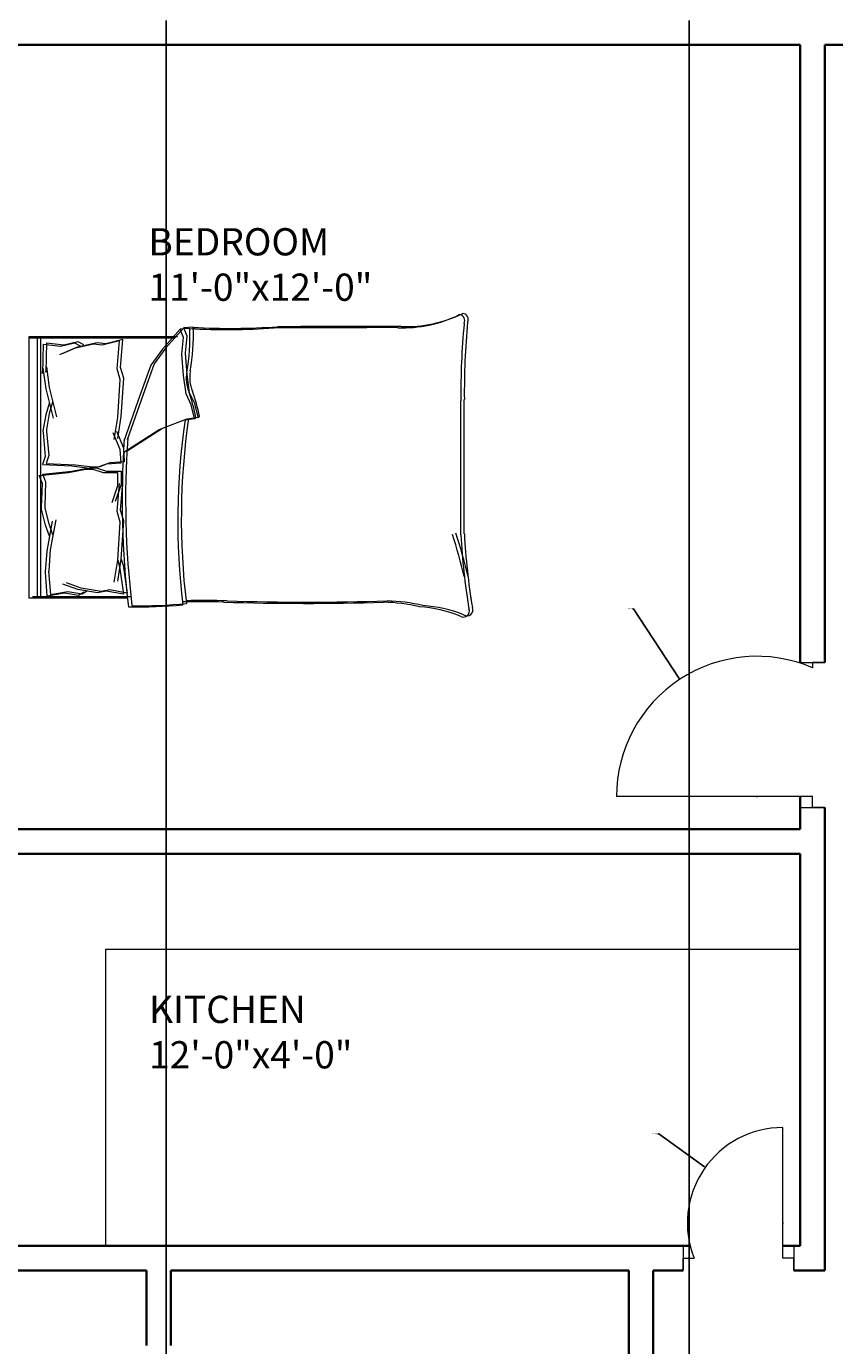
# Model space of a CAD drawing. Units: inches. Extents: x 2163 to 2982, y 1024 to 2288.
# Tile 3 of 22: x 2304 to 2452, y 1395 to 1637. Entities that reach past the tile are written whole.
import ezdxf

# ---------------------------------------------------------------- set-up
doc = ezdxf.new("R2010")
doc.units = ezdxf.units.IN
for name, color, linetype, lineweight in [('A-ANNO-DIMS', 2, 'Continuous', 18), ('A-AREA-IDEN', 7, 'Continuous', 18), ('A-DOOR', 11, 'Continuous', 18), ('A-FLOR-FIXT', 9, 'Continuous', 18), ('A-FURN', 8, 'Continuous', 13), ('A-WALL', 7, 'Continuous', 35)]:
    doc.layers.add(name, color=color, linetype=linetype, lineweight=lineweight)
doc.styles.get("Standard").update_dxf_attribs({"font": 'arial.ttf'})
doc.dimstyles.get("Standard").update_dxf_attribs({"dimtxt": 0.18, "dimasz": 0.18, "dimexe": 0.18, "dimexo": 0.0625, "dimgap": 0.09, "dimtad": 0, "dimtih": 1, "dimtoh": 1, "dimdec": 4, "dimzin": 0, "dimdsep": 46, "dimtxsty": 'Standard', "dimcen": 0.09, "dimadec": 0, "dimazin": 0, "dimtfac": 1, "dimtdec": 4, "dimtofl": 0, "dimtmove": 0, "dimatfit": 3, "dimfxl": 1, "dimtolj": 1, "dimtzin": 0, "dimarcsym": 0})

# ---------------------------------------------------------------- blocks, each defined once
blk = doc.blocks.new('BED-DOUBLE')
for p, q in [((0, 51.49), (0.64, 51.49)), ((0, 3.47), (0, 51.49)), ((0, 51.27), (26.61, 51.27)), ((0, 51.27), (26.61, 51.27)), ((0.64, 51.49), (27.25, 51.49)), ((0.64, 51.49), (27.25, 51.49)), ((1.53, 3.48), (1.53, 51.27)), ((1.53, 3.47), (1.53, 51.27)), ((2.17, 3.7), (2.17, 51.49)), ((2.17, 3.7), (2.17, 51.49)), ((17.21, 50.93), (14.07, 50.15)), ((17.21, 50.93), (14.07, 50.15)), ((16.81, 45.79), (17.21, 50.93)), ((16.81, 45.79), (17.21, 50.93)), ((27.75, 52.87), (24.5, 49.16)), ((27.75, 52.87), (24.5, 49.16)), ((28.38, 53.1), (25.13, 49.39)), ((28.38, 53.1), (25.13, 49.39)), ((29.49, 52.95), (27.75, 52.87, 3.87)), ((29.49, 52.95), (27.75, 52.87, 3.87)), ((28.36, 51.33), (27.75, 52.87)), ((28.36, 51.33), (27.75, 52.87)), ((28.06, 48.23), (28.36, 51.33)), ((28.06, 48.23), (28.36, 51.33)), ((30.13, 53.18), (28.38, 53.1, 3.87)), ((29, 51.56), (28.38, 53.1)), ((30.13, 53.18), (28.38, 53.1, 3.87)), ((29, 51.56), (28.38, 53.1)), ((28.69, 48.46), (29, 51.56)), ((28.69, 48.46), (29, 51.56)), ((2.56, 50.11), (2.46, 44.71)), ((2.56, 50.11), (2.46, 44.71)), ((2.56, 50.11), (5.77, 49.73)), ((2.56, 50.11), (5.77, 49.73)), ((3.2, 50.34), (3.1, 44.94)), ((3.2, 50.34), (3.1, 44.94)), ((3.2, 50.34), (6.41, 49.96)), ((3.2, 50.34), (6.41, 49.96)), ((8.26, 49.31), (5.58, 48.13)), ((8.26, 49.31), (5.58, 48.13)), ((5.77, 49.73), (8.34, 50.33)), ((5.77, 49.73), (8.34, 50.33)), ((8.9, 49.54), (6.22, 48.36)), ((8.9, 49.54), (6.22, 48.36)), ((6.41, 49.96), (8.98, 50.56)), ((6.41, 49.96), (8.98, 50.56)), ((11.83, 50.11), (8.26, 49.31)), ((11.83, 50.11), (8.26, 49.31)), ((8.34, 50.33), (9.38, 49.81)), ((8.34, 50.33), (9.38, 49.81)), ((12.47, 50.34), (8.9, 49.54)), ((12.47, 50.34), (8.9, 49.54)), ((8.98, 50.56), (10.02, 50.04)), ((8.98, 50.56), (10.02, 50.04)), ((13.43, 49.92), (11.83, 50.11)), ((13.43, 49.92), (11.83, 50.11)), ((14.07, 50.15), (12.47, 50.34)), ((14.07, 50.15), (12.47, 50.34)), ((16.57, 50.7), (13.43, 49.92)), ((16.57, 50.7), (13.43, 49.92)), ((16.17, 45.57), (16.57, 50.7)), ((16.17, 45.57), (16.57, 50.7)), ((24.5, 49.16), (22.33, 46.22)), ((24.5, 49.16), (22.33, 46.22)), ((25.13, 49.39), (22.97, 46.45)), ((25.13, 49.39), (22.97, 46.45)), ((29, 44.59), (28.69, 48.46)), ((29, 44.59), (28.69, 48.46)), ((22.33, 46.22), (20.32, 40.64)), ((22.33, 46.22), (20.32, 40.64)), ((22.97, 46.45), (20.96, 40.87)), ((22.97, 46.45), (20.96, 40.87)), ((28.36, 44.36), (28.06, 48.23)), ((28.36, 44.36), (28.06, 48.23)), ((2.46, 44.71), (2.54, 45.71)), ((2.46, 44.71), (2.54, 45.71)), ((2.54, 45.71), (3.07, 41.91)), ((2.54, 45.71), (3.07, 41.91)), ((3.1, 44.94), (3.18, 45.94)), ((3.1, 44.94), (3.18, 45.94)), ((3.18, 45.94), (3.71, 42.14)), ((3.18, 45.94), (3.71, 42.14)), ((16.73, 43.61), (16.17, 45.57)), ((16.73, 43.61), (16.17, 45.57)), ((16.29, 36.6), (16.73, 43.61)), ((16.29, 36.6), (16.73, 43.61)), ((17.37, 43.83), (16.81, 45.79)), ((17.37, 43.83), (16.81, 45.79)), ((16.93, 36.82), (17.37, 43.83)), ((16.93, 36.82), (17.37, 43.83)), ((28.83, 40.95), (28.36, 44.36)), ((28.83, 40.95), (28.36, 44.36)), ((29.47, 41.18), (29, 44.59)), ((29.47, 41.18), (29, 44.59)), ((3.07, 41.91), (4.42, 36.49)), ((3.07, 41.91), (4.42, 36.49)), ((3.71, 42.14), (5.06, 36.72)), ((3.71, 42.14), (5.06, 36.72)), ((30.4, 39.17), (29.47, 41.18)), ((30.4, 39.17), (29.47, 41.18)), ((3.67, 39.2), (3.08, 37.14)), ((3.67, 39.2), (3.08, 37.13)), ((4.31, 39.43), (3.72, 37.36)), ((4.31, 39.43), (3.72, 37.36)), ((20.32, 40.64), (17.38, 32.31)), ((20.32, 40.64), (17.38, 32.31)), ((20.96, 40.87), (18.02, 32.53)), ((20.96, 40.87), (18.02, 32.53)), ((29.76, 38.94), (28.83, 40.95)), ((29.76, 38.94), (28.83, 40.95)), ((30.38, 36.46), (29.76, 38.94)), ((30.38, 36.46), (29.76, 38.94)), ((31.02, 36.69), (30.4, 39.17)), ((31.02, 36.69), (30.4, 39.17)), ((79.24, 15.06), (79.24, 39.68)), ((79.24, 15.06), (79.24, 39.68)), ((79.88, 15.29), (79.88, 39.91)), ((79.88, 15.29), (79.88, 39.91)), ((3.08, 37.14), (2.54, 34.2)), ((3.08, 37.13), (2.54, 34.2)), ((3.72, 37.36), (3.18, 34.43)), ((3.72, 37.36), (3.18, 34.43)), ((15.63, 32.56), (16.29, 36.6)), ((15.63, 32.56), (16.29, 36.6)), ((16.27, 32.79), (16.93, 36.82)), ((16.27, 32.79), (16.93, 36.82)), ((24.52, 34.68), (29, 36.38)), ((24.52, 34.68), (29, 36.38)), ((28.36, 36.15), (30.38, 36.46)), ((28.36, 36.15), (30.38, 36.46)), ((29, 36.38), (31.02, 36.69)), ((29, 36.38), (31.02, 36.69)), ((2.54, 34.2), (2.56, 33.88)), ((2.54, 34.2), (2.56, 33.88)), ((3.18, 34.43), (3.2, 34.11)), ((3.18, 34.43), (3.2, 34.11)), ((3.2, 34.11), (3.62, 29.68)), ((3.2, 34.11), (3.62, 29.68)), ((17.38, 30.98), (16.09, 34.05)), ((17.38, 30.98), (16.09, 34.05)), ((17.38, 30.26), (23.88, 34.45)), ((17.38, 30.26), (23.88, 34.45)), ((18.02, 30.49), (24.52, 34.68)), ((18.02, 30.49), (24.52, 34.68)), ((23.88, 34.45), (28.36, 36.15)), ((23.88, 34.45), (28.36, 36.15)), ((2.56, 33.88), (2.98, 29.46)), ((2.56, 33.88), (2.98, 29.46)), ((16.74, 30.75), (15.45, 33.82)), ((16.74, 30.75), (15.45, 33.82)), ((2.98, 29.46), (2.49, 27.98)), ((2.98, 29.46), (2.49, 27.98)), ((3.62, 29.68), (3.13, 28.21)), ((3.62, 29.68), (3.13, 28.2)), ((16.89, 28.3), (16.74, 30.75)), ((16.89, 28.3), (16.74, 30.75)), ((17.53, 28.53), (17.38, 30.98)), ((17.53, 28.53), (17.38, 30.98)), ((2.49, 27.98), (7.87, 27.73)), ((2.49, 27.98), (7.87, 27.73)), ((2.51, 26.21), (7.86, 26.79)), ((2.51, 26.21), (7.86, 26.79)), ((3.13, 28.21), (8.51, 27.96)), ((3.13, 28.2), (8.51, 27.96)), ((7.22, 26.56), (10.4, 27.14)), ((7.22, 26.56), (10.4, 27.14)), ((7.86, 26.79), (11.04, 27.37)), ((7.86, 26.79), (11.04, 27.37)), ((7.87, 27.73), (11.08, 27.35)), ((7.87, 27.73), (11.08, 27.35)), ((8.51, 27.96), (11.72, 27.58)), ((8.51, 27.96), (11.72, 27.58)), ((10.4, 27.14), (11.7, 27.14)), ((10.4, 27.14), (11.7, 27.14)), ((11.04, 27.37), (12.34, 27.37)), ((11.04, 27.37), (12.34, 27.37)), ((11.08, 27.35), (12.38, 27.44)), ((11.08, 27.35), (12.38, 27.44)), ((11.7, 27.14), (13.58, 26.56)), ((11.7, 27.14), (13.58, 26.56)), ((11.72, 27.58), (13.02, 27.66)), ((11.72, 27.58), (13.02, 27.66)), ((12.34, 27.37), (14.22, 26.79)), ((12.34, 27.37), (14.22, 26.79)), ((12.38, 27.44), (14.22, 28.13)), ((12.38, 27.44), (14.22, 28.13)), ((13.02, 27.66), (14.86, 28.36)), ((13.02, 27.66), (14.86, 28.36)), ((14.22, 28.13), (16.89, 28.3)), ((14.22, 28.13), (16.89, 28.3)), ((14.22, 26.79), (16.9, 26.79)), ((14.22, 26.79), (16.9, 26.79)), ((14.86, 28.36), (17.53, 28.53)), ((14.86, 28.36), (17.53, 28.53)), ((16.9, 26.79), (16.9, 24.33)), ((16.9, 26.79), (16.9, 24.33)), ((1.87, 25.98), (7.22, 26.56)), ((1.87, 25.98), (7.22, 26.56)), ((2.45, 24.54), (1.87, 25.98)), ((2.45, 24.54), (1.87, 25.98)), ((2.3, 20.09), (2.45, 24.54)), ((2.3, 20.09), (2.45, 24.54)), ((3.09, 24.77), (2.51, 26.21)), ((3.09, 24.77), (2.51, 26.21)), ((2.94, 20.32), (3.09, 24.77)), ((2.94, 20.32), (3.09, 24.77)), ((13.58, 26.56), (16.26, 26.56)), ((13.58, 26.56), (16.26, 26.56)), ((16.9, 24.33), (15.81, 21.19)), ((16.9, 24.33), (15.81, 21.19)), ((16.17, 19.38), (16.57, 24.52)), ((16.17, 19.38), (16.57, 24.52)), ((16.26, 26.56), (16.26, 24.1)), ((16.26, 26.56), (16.26, 24.1)), ((16.81, 19.61), (17.21, 24.74)), ((16.81, 19.61), (17.21, 24.74)), ((16.26, 24.1), (15.17, 20.96)), ((16.26, 24.1), (15.17, 20.96)), ((2.3, 19.77), (2.3, 20.09)), ((2.3, 19.77), (2.3, 20.09)), ((3.03, 16.88), (2.3, 19.77)), ((3.03, 16.88), (2.3, 19.77)), ((2.94, 20), (2.94, 20.32)), ((2.94, 20), (2.94, 20.32)), ((3.67, 17.11), (2.94, 20)), ((3.67, 17.11), (2.94, 20)), ((16.73, 17.42), (16.17, 19.38)), ((16.73, 17.42), (16.17, 19.38)), ((17.37, 17.65), (16.81, 19.61)), ((17.37, 17.65), (16.81, 19.61)), ((3.32, 12.11), (4.33, 17.6)), ((3.32, 12.11), (4.33, 17.6)), ((4.39, 15.08), (3.67, 17.11)), ((4.39, 15.08), (3.67, 17.11)), ((3.96, 12.34), (4.97, 17.83)), ((3.96, 12.34), (4.97, 17.83)), ((16.29, 10.41), (16.73, 17.42)), ((16.29, 10.41), (16.73, 17.42)), ((16.93, 10.64), (17.37, 17.65)), ((16.93, 10.64), (17.37, 17.65)), ((3.75, 14.85), (3.03, 16.88)), ((3.75, 14.85), (3.03, 16.88)), ((3.03, 8.28), (3.32, 12.11)), ((3.67, 8.51), (3.96, 12.34)), ((3.67, 8.51), (3.96, 12.34)), ((3.03, 8.28), (3.32, 12.11)), ((15.63, 6.38), (16.29, 10.41)), ((15.63, 6.38), (16.29, 10.41)), ((16.27, 6.61), (16.93, 10.64)), ((16.27, 6.61), (16.93, 10.64)), ((16.29, 10.41), (16.62, 9.28)), ((16.29, 10.41), (16.62, 9.28)), ((16.93, 10.64), (17.26, 9.51)), ((16.93, 10.64), (17.26, 9.51)), ((3.01, 8.18), (3.03, 8.28)), ((3.01, 8.18), (3.03, 8.28)), ((3.34, 3.9), (3.01, 8.18)), ((3.34, 3.9), (3.01, 8.18)), ((3.65, 8.41), (3.67, 8.51)), ((3.65, 8.41), (3.67, 8.51)), ((3.98, 4.13), (3.65, 8.41)), ((3.98, 4.13), (3.65, 8.41)), ((16.62, 9.28), (17.34, 4.18)), ((16.62, 9.28), (17.34, 4.18)), ((17.26, 9.51), (17.98, 4.41)), ((17.26, 9.51), (17.98, 4.41)), ((8.95, 5.05), (6.21, 6.06)), ((8.95, 5.05), (6.21, 6.06)), ((9.59, 5.28), (6.85, 6.29)), ((9.59, 5.28), (6.85, 6.29)), ((12.57, 4.47), (8.95, 5.05)), ((12.57, 4.47), (8.95, 5.05)), ((13.21, 4.7), (9.59, 5.28)), ((13.21, 4.7), (9.59, 5.28)), ((9.74, 4.27), (10.75, 4.85)), ((9.74, 4.27), (10.75, 4.85)), ((14.8, 4.99), (13.21, 4.7)), ((14.8, 4.99), (13.21, 4.7)), ((17.98, 4.41), (14.8, 4.99)), ((17.98, 4.41), (14.8, 4.99)), ((18.11, 3.48), (0, 3.48)), ((18.11, 3.47), (0, 3.47)), ((18.75, 3.7), (0.64, 3.7)), ((18.75, 3.7), (0.64, 3.7)), ((3.32, 3.89), (6.5, 4.47)), ((3.32, 3.89), (6.5, 4.47)), ((3.96, 4.12), (7.14, 4.7)), ((3.96, 4.12), (7.14, 4.7)), ((6.5, 4.47), (9.1, 4.04)), ((6.5, 4.47), (9.1, 4.04)), ((7.14, 4.7), (9.74, 4.27)), ((7.14, 4.7), (9.74, 4.27)), ((9.1, 4.04), (10.11, 4.62)), ((9.1, 4.04), (10.11, 4.62)), ((14.16, 4.76), (12.57, 4.47)), ((14.16, 4.76), (12.57, 4.47)), ((17.34, 4.18), (14.16, 4.76)), ((17.34, 4.18), (14.16, 4.76))]:
    blk.add_line(p, q)
for centre, radius, start, end in [((69.31, 76.39), 23.07, 267.4714, 296.4681), ((69.31, 76.39), 23.07, 267.4714, 296.4681), ((79.51, 54.64), 1.1, 332.6588, 86.02), ((79.51, 54.64), 1.1, 332.6588, 86.02), ((36.95, 182.49), 129.5, 266.9791, 273.8365), ((36.95, 182.49), 129.5, 266.9791, 273.8365), ((68.46, -4508.52), 4561.86, 90.00217, 90.28689), ((68.46, -4508.52), 4561.86, 90.00217, 90.28689), ((68.67, 76.16), 23.07, 267.4714, 296.4681), ((68.67, 76.16), 23.07, 267.4714, 296.4681), ((78.87, 54.41), 1.1, 332.6588, 86.02), ((78.87, 54.41), 1.1, 332.6588, 86.02), ((212.28, 41.15), 133.04, 174.4998, 180.6351), ((212.28, 41.15), 133.04, 174.4998, 180.6351), ((212.92, 41.38), 133.04, 174.4998, 180.6351), ((212.92, 41.38), 133.04, 174.4998, 180.6351), ((-6.66, 51.33), 36.18, 349.8763, 2.5657), ((-6.66, 51.33), 36.18, 349.8763, 2.5657), ((36.31, 182.27), 129.5, 266.9791, 273.8365), ((36.31, 182.27), 129.5, 266.9791, 273.8365), ((-6.02, 51.56), 36.18, 349.8763, 2.5657), ((-6.02, 51.56), 36.18, 349.8763, 2.5657), ((67.82, -4508.74), 4561.86, 90.00217, 90.28689), ((67.82, -4508.74), 4561.86, 90.00217, 90.28689), ((35.07, 43.74), 6.22, 168.6608, 203.7384), ((35.07, 43.74), 6.22, 168.6608, 203.7384), ((35.71, 43.97), 6.22, 168.6608, 203.7384), ((35.71, 43.97), 6.22, 168.6608, 203.7384), ((1.48, 31.15), 29.65, 10.6617, 19.8806), ((1.48, 31.15), 29.65, 10.6617, 19.8806), ((2.12, 31.38), 29.65, 10.6617, 19.8806), ((2.12, 31.38), 29.65, 10.6617, 19.8806), ((156.96, 17.98), 129.02, 171.7845, 186.9006), ((156.96, 17.98), 129.02, 171.7845, 186.9006), ((30.44, 36.64), 0.185, 250.2464, 1.1377), ((30.44, 36.64), 0.185, 250.2464, 1.1377), ((31.08, 36.86), 0.185, 250.2464, 1.1377), ((31.08, 36.86), 0.185, 250.2464, 1.1377), ((156.32, 17.76), 129.02, 171.7845, 186.9006), ((156.32, 17.76), 129.02, 171.7845, 186.9006), ((182.05, 21.36), 164.97, 176.0865, 186.7821), ((182.05, 21.36), 164.97, 176.0865, 186.7821), ((182.69, 21.59), 164.97, 176.0865, 186.7821), ((182.69, 21.59), 164.97, 176.0865, 186.7821), ((-23.71, -17.22), 106.46, 13.3832, 17.7053), ((-23.71, -17.22), 106.46, 13.3832, 17.7053), ((-23.07, -16.99), 106.46, 13.3832, 17.7053), ((-23.07, -16.99), 106.46, 13.3832, 17.7053), ((200.84, 21.43), 121.76, 182.9958, 189.4091), ((200.84, 21.43), 121.76, 182.9958, 189.4091), ((201.48, 21.66), 121.76, 182.9958, 189.4091), ((201.48, 21.65), 121.76, 182.9958, 189.4091), ((20.74, 85.39), 83.31, 268.7218, 275.604), ((20.74, 85.39), 83.31, 268.7218, 275.604), ((31.17, -167.31), 170.11, 88.4762, 91.0082), ((31.17, -167.31), 170.11, 88.4762, 91.0082), ((31.81, -167.08), 170.11, 88.4762, 91.0082), ((31.81, -167.08), 170.11, 88.4762, 91.0082), ((50.61, 484.82), 482.31, 268.2277, 271.7185), ((50.61, 484.82), 482.31, 268.2277, 271.7185), ((51.25, 485.05), 482.31, 268.2277, 271.7185), ((51.25, 485.05), 482.31, 268.2277, 271.7185), ((64.51, -26.9), 29.63, 76.0648, 88.9113), ((64.51, -26.9), 29.63, 76.0648, 88.9113), ((65.15, -26.67), 29.63, 76.0648, 88.9113), ((65.15, -26.67), 29.63, 76.0648, 88.9113), ((20.1, 85.16), 83.31, 268.7218, 275.604), ((20.1, 85.16), 83.31, 268.7218, 275.604), ((70.28, -21.66), 23.56, 67.9751, 86.652), ((70.28, -21.66), 23.56, 67.9751, 86.652), ((70.91, -21.43), 23.56, 67.9751, 86.652), ((70.91, -21.43), 23.56, 67.9751, 86.652), ((79.72, 1.09), 1.09, 236.1736, 23.4781), ((79.72, 1.09), 1.09, 236.1736, 23.4781), ((80.36, 1.32), 1.09, 236.1736, 23.4781), ((80.36, 1.32), 1.09, 236.1736, 23.4781)]:
    blk.add_arc(centre, radius, start, end)
blk = doc.blocks.new('*D36')
at = {"layer": 'A-ANNO-DIMS', "color": 0, "lineweight": -2, "transparency": 16777216}
for p, q in [((2289.84, 1638.21), (2289.84, 1023.79)), ((2329.44, 1638.21), (2329.44, 1023.79)), ((2290.02, 1023.97), (2309.18, 1023.97)), ((2329.26, 1023.97), (2310.11, 1023.97))]:
    blk.add_line(p, q, dxfattribs=at)
at = {"layer": 'A-ANNO-DIMS', "color": 0, "transparency": 16777216}
for points in [[(2290.02, 1024), (2290.02, 1023.94), (2289.84, 1023.97)], [(2329.26, 1024), (2329.26, 1023.94), (2329.44, 1023.97)]]:
    blk.add_solid(points, dxfattribs=at)
at = {"layer": 'Defpoints', "color": 0, "transparency": 16777216}
for p in [(2289.84, 1638.27), (2329.44, 1638.27), (2329.44, 1023.97)]:
    blk.add_point(p, dxfattribs=at)
at = {"layer": 'A-ANNO-DIMS', "color": 0, "transparency": 16777216, "insert": (2309.64, 1023.97), "char_height": 0.18, "attachment_point": 5}
blk.add_mtext('\\A1;39.605', dxfattribs=at)
blk = doc.blocks.new('*D37')
at = {"layer": 'A-ANNO-DIMS', "color": 0, "lineweight": -2, "transparency": 16777216}
for p, q in [((2329.44, 1638.21), (2329.44, 1023.79)), ((2425.44, 1638.21), (2425.44, 1023.79)), ((2329.62, 1023.97), (2377.22, 1023.97)), ((2425.26, 1023.97), (2377.66, 1023.97))]:
    blk.add_line(p, q, dxfattribs=at)
at = {"layer": 'A-ANNO-DIMS', "color": 0, "transparency": 16777216}
for points in [[(2329.62, 1024), (2329.62, 1023.94), (2329.44, 1023.97)], [(2425.26, 1024), (2425.26, 1023.94), (2425.44, 1023.97)]]:
    blk.add_solid(points, dxfattribs=at)
at = {"layer": 'Defpoints', "color": 0, "transparency": 16777216}
for p in [(2329.44, 1638.27), (2425.44, 1638.27), (2425.44, 1023.97)]:
    blk.add_point(p, dxfattribs=at)
at = {"layer": 'A-ANNO-DIMS', "color": 0, "transparency": 16777216, "insert": (2377.44, 1023.97), "char_height": 0.18, "attachment_point": 5}
blk.add_mtext('\\A1;96', dxfattribs=at)
blk = doc.blocks.new('*D54')
at = {"layer": 'A-ANNO-DIMS', "color": 0, "lineweight": -2, "transparency": 16777216}
for p, q in [((2415.04, 1530.21), (2415.22, 1530.21)), ((2415.22, 1530.21), (2423.61, 1517.44)), ((2437.77, 1495.75), (2437.95, 1495.75)), ((2437.86, 1495.66), (2437.86, 1495.84))]:
    blk.add_line(p, q, dxfattribs=at)
at = {"layer": 'A-ANNO-DIMS', "color": 0, "transparency": 16777216}
blk.add_solid([(2423.64, 1517.45), (2423.58, 1517.42), (2423.71, 1517.29)], dxfattribs=at)
at = {"layer": 'Defpoints', "color": 0, "transparency": 16777216}
for p in [(2423.71, 1517.29), (2437.86, 1495.75)]:
    blk.add_point(p, dxfattribs=at)
at = {"layer": 'A-ANNO-DIMS', "color": 0, "transparency": 16777216, "insert": (2414.56, 1530.21), "char_height": 0.18, "attachment_point": 5}
blk.add_mtext('\\A1;R25.77', dxfattribs=at)
blk = doc.blocks.new('*D75')
at = {"layer": 'A-ANNO-DIMS', "color": 0, "lineweight": -2, "transparency": 16777216}
for p, q in [((2419.68, 1433.84), (2419.86, 1433.84)), ((2419.86, 1433.84), (2428.25, 1427.82)), ((2442.54, 1417.5), (2442.72, 1417.5)), ((2442.63, 1417.41), (2442.63, 1417.59))]:
    blk.add_line(p, q, dxfattribs=at)
at = {"layer": 'A-ANNO-DIMS', "color": 0, "transparency": 16777216}
blk.add_solid([(2428.27, 1427.84), (2428.23, 1427.79), (2428.4, 1427.71)], dxfattribs=at)
at = {"layer": 'Defpoints', "color": 0, "transparency": 16777216}
for p in [(2428.4, 1427.71), (2442.63, 1417.5)]:
    blk.add_point(p, dxfattribs=at)
at = {"layer": 'A-ANNO-DIMS', "color": 0, "transparency": 16777216, "insert": (2419.13, 1433.84), "char_height": 0.18, "attachment_point": 5}
blk.add_mtext('\\A1;R17.518', dxfattribs=at)

msp = doc.modelspace()

# ---------------------------------------------------------------- linework, layer by layer
at = {"layer": 'A-DOOR'}
for p, q in [((2445.8389, 1520.3989), (2450.3389, 1520.3989)), ((2450.3389, 1520.3989), (2448.0889, 1520.3989)), ((2448.0889, 1520.3989), (2448.0889, 1519.3989)), ((2448.0889, 1495.7484), (2412.0889, 1495.7484)), ((2448.0889, 1493.7484), (2448.0889, 1495.7484)), ((2445.8389, 1493.7484), (2450.3389, 1493.7484)), ((2450.3389, 1493.7484), (2448.0889, 1493.7484)), ((2442.6306, 1411.0188), (2442.6306, 1435.0188)), ((2424.3566, 1413.2688), (2424.3566, 1408.7688)), ((2444.6306, 1413.2688), (2444.6306, 1408.7688)), ((2424.3566, 1408.7688), (2424.3566, 1411.0188)), ((2424.3566, 1411.0188), (2426.3566, 1411.0188)), ((2444.6306, 1411.0188), (2442.6306, 1411.0188)), ((2444.6306, 1408.7688), (2444.6306, 1411.0188))]:
    msp.add_line(p, q, dxfattribs=at)
for centre, radius, start, end in [((2437.8576, 1495.7484), 25.7687, 66.606476, 180), ((2442.6306, 1417.5013), 17.5176, 90, 201.718944)]:
    msp.add_arc(centre, radius, start, end, dxfattribs=at)
at = {"layer": 'A-FLOR-FIXT'}
for p, q in [((2318.3613, 1413.2688), (2318.3613, 1467.7598)), ((2318.3613, 1467.7598), (2445.8389, 1467.7598))]:
    msp.add_line(p, q, dxfattribs=at)
at = {"layer": 'A-WALL'}
for p, q in [((2301.8389, 1633.7688), (2445.8389, 1633.7688)), ((2445.8389, 1633.7688), (2445.8389, 1520.2499)), ((2450.3389, 1633.7688), (2450.3389, 1520.3989)), ((2450.3389, 1633.7688), (2455.9219, 1633.7688)), ((2445.8389, 1495.7484), (2445.8389, 1489.7688)), ((2450.3389, 1493.7484), (2450.3389, 1408.7688)), ((2301.8389, 1489.7688), (2445.8389, 1489.7688)), ((2301.8389, 1485.2688), (2445.8389, 1485.2688)), ((2445.8389, 1485.2688), (2445.8389, 1413.2688)), ((2301.8389, 1413.2688), (2425.632, 1413.2688)), ((2442.6306, 1413.2688), (2445.8389, 1413.2688)), ((2297.3389, 1408.7688), (2325.8389, 1408.7688)), ((2325.8389, 1408.7688), (2325.8389, 1394.9788)), ((2330.3389, 1408.7688), (2330.3389, 1394.9788)), ((2330.3389, 1408.7688), (2414.3389, 1408.7688)), ((2414.3389, 1408.7688), (2414.3389, 1377.1151)), ((2418.8389, 1408.7688), (2418.8389, 1378.2153)), ((2418.8389, 1408.7688), (2424.3566, 1408.7688)), ((2444.6306, 1408.7688), (2450.3389, 1408.7688))]:
    msp.add_line(p, q, dxfattribs=at)

# ---------------------------------------------------------------- block references
at = {"layer": 'A-FURN'}
msp.add_blockref('BED-DOUBLE', (2304.2965, 1528.7218), dxfattribs=at)

# ---------------------------------------------------------------- texts
at = {"layer": 'A-AREA-IDEN', "char_height": 5, "attachment_point": 1}
for s, width, insert in [('BEDROOM\\P11\'-0"x12\'-0"', 80.429198, (2326.1949, 1600.1029)), ('KITCHEN\\P12\'-0"x4\'-0"', 82.635303, (2326.3204, 1459.2013))]:
    msp.add_mtext_dynamic_manual_height_columns(s, width=width, gutter_width=12.5, heights=[0], dxfattribs=dict(at, insert=insert))

# ---------------------------------------------------------------- dimensions: what is measured, and where the dimension line sits
at = {"layer": 'A-ANNO-DIMS'}
for base, p1, p2, override, picture, middle in [((2329.44344, 1023.97342), (2289.83891, 1638.26884), (2329.44344, 1638.26884), {"dimdec": 3, "dimlfac": 1, "dimrnd": 0, "dimzin": 0, "dimdsep": 46, "dimlunit": 2}, '*D36', (2309.64118, 1023.97342)), ((2425.4434, 1023.9734), (2329.4434, 1638.2688), (2425.4434, 1638.2688), {"dimdec": 0, "dimlfac": 1, "dimrnd": 0, "dimzin": 0, "dimdsep": 46, "dimlunit": 2}, '*D37', (2377.4434, 1023.9734))]:
    dim = msp.add_linear_dim(base=base, p1=p1, p2=p2, dimstyle='Standard', override=override, dxfattribs=at)
    dim.commit()
    dim.dimension.update_dxf_attribs({"geometry": picture, "text_midpoint": middle})
for center, mpoint, override, picture, middle in [((2437.8576, 1495.7484), (2423.7088, 1517.2853), {"dimdec": 2, "dimlfac": 1, "dimrnd": 0, "dimzin": 0, "dimdsep": 46, "dimlunit": 2}, '*D54', (2414.5597, 1530.2074)), ((2442.6306, 1417.5013), (2428.3982, 1427.7142), {"dimdec": 3, "dimlfac": 1, "dimrnd": 0, "dimzin": 0, "dimdsep": 46, "dimlunit": 2}, '*D75', (2419.1288, 1433.842))]:
    dim = msp.add_radius_dim(center=center, mpoint=mpoint, dimstyle='Standard', override=override, dxfattribs=at)
    dim.commit()
    dim.dimension.update_dxf_attribs({"geometry": picture, "text_midpoint": middle, "dimtype": 164})

doc.saveas('drawing.dxf')
